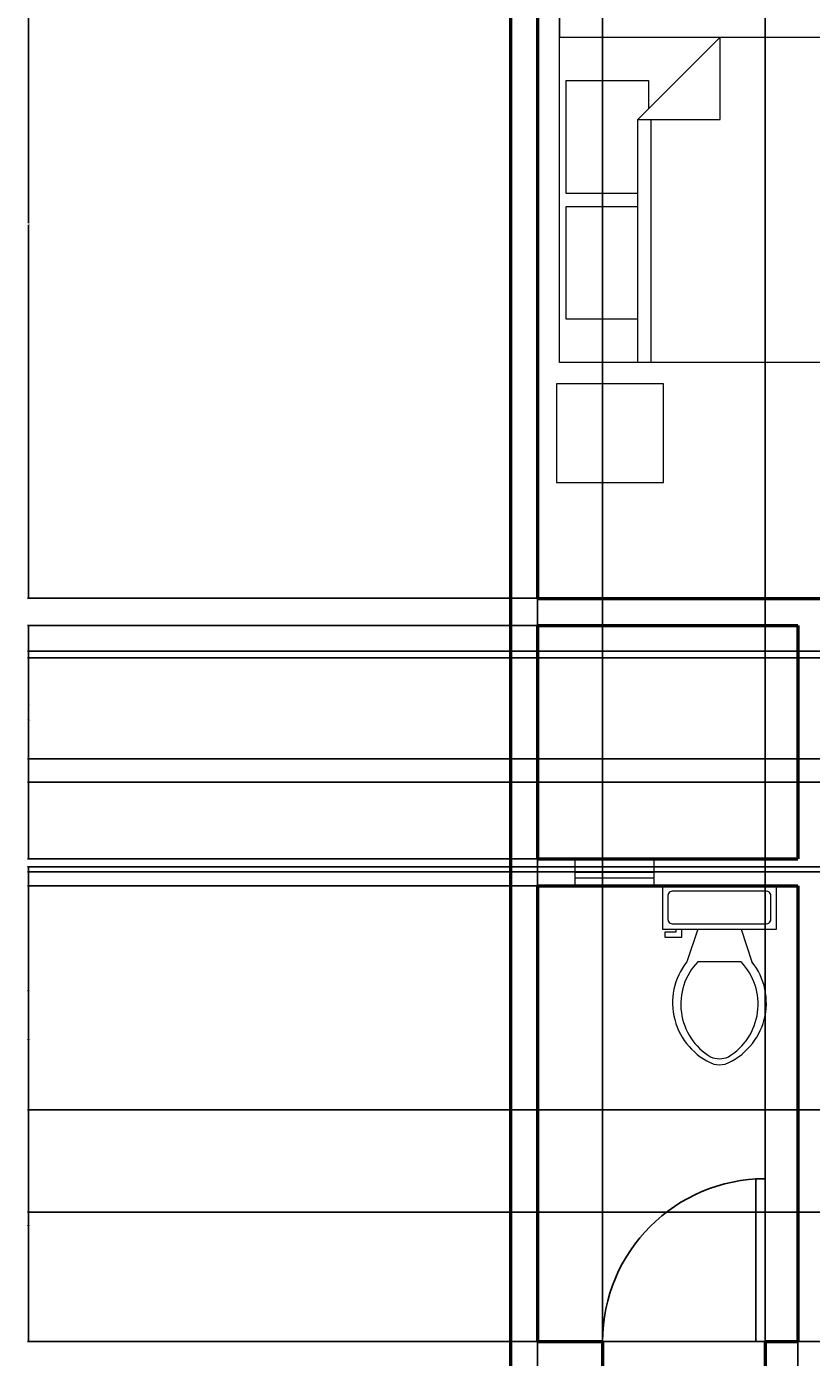
# Model space of a CAD drawing. Units: inches. Extents: x 115999 to 116502, y 188991 to 189729.
# Tile 2 of 5: x 115999 to 116144, y 189347 to 189592. Entities that reach past the tile are written whole.
import ezdxf

# ---------------------------------------------------------------- set-up
doc = ezdxf.new("R2010")
doc.units = ezdxf.units.IN
for name, color, linetype, lineweight in [('A-ANNO-DIMS', 2, 'Continuous', 18), ('A-DOOR', 4, 'Continuous', 25), ('A-FLOR-FIXT', 9, 'Continuous', 20), ('A-FURN', 8, 'Continuous', 18), ('A-GLAZ', 4, 'Continuous', 18), ('A-WALL', 7, 'Continuous', 50)]:
    doc.layers.add(name, color=color, linetype=linetype, lineweight=lineweight)
doc.styles.get("Standard").update_dxf_attribs({"font": 'arial.ttf'})
doc.dimstyles.get("Standard").update_dxf_attribs({"dimtxt": 0.18, "dimasz": 0.18, "dimexe": 0.18, "dimexo": 0.0625, "dimgap": 0.09, "dimtad": 0, "dimtih": 1, "dimtoh": 1, "dimdec": 4, "dimzin": 0, "dimdsep": 46, "dimtxsty": 'Standard', "dimcen": 0.09, "dimadec": 0, "dimazin": 0, "dimtfac": 1, "dimtdec": 4, "dimtofl": 0, "dimtmove": 0, "dimatfit": 3, "dimfxl": 1, "dimtolj": 1, "dimtzin": 0, "dimarcsym": 0})

# ---------------------------------------------------------------- blocks, each defined once
blk = doc.blocks.new('Toilet - top')
for p, q in [((9.5, -6), (9.5, -2)), ((-10, -8.5), (-8, -8.5)), ((-10, -9.5), (-10, -8.5)), ((-7, -9.5), (-10, -9.5)), ((-8, -8.5), (-8, -8)), ((-7, -8), (-7, -9.5)), ((-4, -8), (-6, -14)), ((4, -8), (6, -14)), ((4, -14), (-4, -14))]:
    blk.add_line(p, q)
blk.add_lwpolyline([(10.5, -8), (10.5, 0), (-10.5, 0), (-10.5, -8)], close=True)
for points in [[(-9.5, -2), (-9.5, -6)], [(8.5, -1), (-8.5, -1)], [(-8.5, -7), (8.5, -7)]]:
    blk.add_lwpolyline(points)
for centre, radius, start, end in [((-8.62, -1.88), 0.884, 81.8699, 188.1301), ((8.62, -1.88), 0.884, 351.8699, 98.1301), ((-8.62, -6.12), 0.884, 171.8699, 278.1301), ((8.62, -6.12), 0.884, 261.8699, 8.1301), ((3.52, -21.58), 12.17, 141.4691, 247.9714), ((4.2, -21.82), 11.33, 136.3677, 238.9468), ((-3.52, -21.58), 12.17, 292.0284, 38.5307), ((-4.2, -21.82), 11.33, 301.053, 43.6321), ((0, -27.88), 4, 245.7318, 294.2682), ((0, -29), 4, 254.8605, 285.1395)]:
    blk.add_arc(centre, radius, start, end)
blk = doc.blocks.new('Bed - Queen')
for p, q in [((0, -80.00003), (0, 0)), ((0, 0), (59.99999, 0)), ((59.99999, 0), (59.99999, -80.00003)), ((7.99999, -1.2), (28.79998, -1.2)), ((7.99999, -14.4), (7.99999, -1.2)), ((28.79998, -1.2), (28.79998, -14.4)), ((31.19999, -1.2), (51.99999, -1.2)), ((31.19999, -14.4), (31.19999, -1.2)), ((51.99999, -1.2), (51.99999, -16.4)), ((0, -14.4), (44.8, -14.4)), ((59.99999, -29.6), (44.8, -14.4)), ((44.8, -14.4), (44.8, -29.6)), ((44.8, -16.8), (0, -16.8)), ((51.99999, -16.4), (46.79936, -16.4)), ((44.8, -29.6), (59.99999, -29.6)), ((59.99999, -80.00003), (0, -80.00003))]:
    blk.add_line(p, q)
blk = doc.blocks.new('*U3')
for p, q in [((0, 0), (0, -5)), ((30, 0), (30, -5))]:
    blk.add_line(p, q)
blk.add_lwpolyline([(0, 0), (0, 30), (1.75, 30), (1.75, 0)], close=True)
blk.add_arc((0, 0), 30, 0, 90)
blk = doc.blocks.new('TABLE-NIGHTSTAND')
blk.add_lwpolyline([(0, 18.2), (19.71, 18.2), (19.71, 0), (0, 0)], close=True)
blk = doc.blocks.new('*D21')
at = {"layer": 'A-ANNO-DIMS', "color": 0, "lineweight": -2, "transparency": 16777216}
for p, q in [((116097.14, 189590.46), (116097.14, 189602.58)), ((116097.32, 189602.4), (116135.84, 189602.4)), ((116176.96, 189602.4), (116138.45, 189602.4)), ((116177.14, 189590.46), (116177.14, 189602.58))]:
    blk.add_line(p, q, dxfattribs=at)
at = {"layer": 'A-ANNO-DIMS', "color": 0, "transparency": 16777216}
for points in [[(116097.32, 189602.43), (116097.32, 189602.37), (116097.14, 189602.4)], [(116176.96, 189602.43), (116176.96, 189602.37), (116177.14, 189602.4)]]:
    blk.add_solid(points, dxfattribs=at)
at = {"layer": 'Defpoints', "color": 0, "transparency": 16777216}
for p in [(116097.14, 189602.4), (116097.14, 189590.4), (116177.14, 189590.4)]:
    blk.add_point(p, dxfattribs=at)
at = {"layer": 'A-ANNO-DIMS', "color": 0, "transparency": 16777216, "insert": (116137.14, 189602.4), "char_height": 0.18, "attachment_point": 5}
blk.add_mtext('\\A1;QUEEN BED 80 TYP.', dxfattribs=at)
blk = doc.blocks.new('*D33')
at = {"layer": 'A-ANNO-DIMS', "color": 0, "lineweight": -2, "transparency": 16777216}
for p, q in [((116088.06, 189088.01), (116088.06, 189728.73)), ((116088.24, 189728.55), (116277.77, 189728.55)), ((116467.88, 189728.55), (116278.35, 189728.55)), ((116468.06, 189088.01), (116468.06, 189728.73))]:
    blk.add_line(p, q, dxfattribs=at)
at = {"layer": 'A-ANNO-DIMS', "color": 0, "transparency": 16777216}
for points in [[(116088.24, 189728.58), (116088.24, 189728.52), (116088.06, 189728.55)], [(116467.88, 189728.58), (116467.88, 189728.52), (116468.06, 189728.55)]]:
    blk.add_solid(points, dxfattribs=at)
at = {"layer": 'Defpoints', "color": 0, "transparency": 16777216}
for p in [(116468.06, 189728.55), (116088.06, 189087.95), (116468.06, 189087.95)]:
    blk.add_point(p, dxfattribs=at)
at = {"layer": 'A-ANNO-DIMS', "color": 0, "transparency": 16777216, "insert": (116278.06, 189728.55), "char_height": 0.18, "attachment_point": 5}
blk.add_mtext('\\A1;380', dxfattribs=at)
blk = doc.blocks.new('*D39')
at = {"layer": 'A-ANNO-DIMS', "color": 0, "lineweight": -2, "transparency": 16777216}
for p, q in [((116093, 189624.95), (115999.04, 189624.95)), ((115999.22, 189624.77), (115999.22, 189556.13)), ((115999.22, 189487.13), (115999.22, 189555.76)), ((116093, 189486.95), (115999.04, 189486.95))]:
    blk.add_line(p, q, dxfattribs=at)
at = {"layer": 'A-ANNO-DIMS', "color": 0, "transparency": 16777216}
for points in [[(115999.19, 189624.77), (115999.25, 189624.77), (115999.22, 189624.95)], [(115999.19, 189487.13), (115999.25, 189487.13), (115999.22, 189486.95)]]:
    blk.add_solid(points, dxfattribs=at)
at = {"layer": 'Defpoints', "color": 0, "transparency": 16777216}
for p in [(115999.22, 189624.95), (116093.06, 189624.95), (116093.06, 189486.95)]:
    blk.add_point(p, dxfattribs=at)
at = {"layer": 'A-ANNO-DIMS', "color": 0, "transparency": 16777216, "insert": (115999.22, 189555.95), "char_height": 0.18, "attachment_point": 5}
blk.add_mtext('\\A1;138', dxfattribs=at)
blk = doc.blocks.new('*D41')
at = {"layer": 'A-ANNO-DIMS', "color": 0, "lineweight": -2, "transparency": 16777216}
for p, q in [((116093, 189433.95), (115999.04, 189433.95)), ((115999.22, 189433.77), (115999.22, 189392.13)), ((115999.22, 189350.13), (115999.22, 189391.77)), ((116093, 189349.95), (115999.04, 189349.95))]:
    blk.add_line(p, q, dxfattribs=at)
at = {"layer": 'A-ANNO-DIMS', "color": 0, "transparency": 16777216}
for points in [[(115999.19, 189433.77), (115999.25, 189433.77), (115999.22, 189433.95)], [(115999.19, 189350.13), (115999.25, 189350.13), (115999.22, 189349.95)]]:
    blk.add_solid(points, dxfattribs=at)
at = {"layer": 'Defpoints', "color": 0, "transparency": 16777216}
for p in [(115999.22, 189433.95), (116093.06, 189433.95), (116093.06, 189349.95)]:
    blk.add_point(p, dxfattribs=at)
at = {"layer": 'A-ANNO-DIMS', "color": 0, "transparency": 16777216, "insert": (115999.22, 189391.95), "char_height": 0.18, "attachment_point": 5}
blk.add_mtext('\\A1;84', dxfattribs=at)
blk = doc.blocks.new('*D42')
at = {"layer": 'A-ANNO-DIMS', "color": 0, "lineweight": -2, "transparency": 16777216}
for p, q in [((116093, 189481.95), (115999.04, 189481.95)), ((115999.22, 189481.77), (115999.22, 189460.63)), ((115999.22, 189439.13), (115999.22, 189460.26)), ((116093, 189438.95), (115999.04, 189438.95))]:
    blk.add_line(p, q, dxfattribs=at)
at = {"layer": 'A-ANNO-DIMS', "color": 0, "transparency": 16777216}
for points in [[(115999.19, 189481.77), (115999.25, 189481.77), (115999.22, 189481.95)], [(115999.19, 189439.13), (115999.25, 189439.13), (115999.22, 189438.95)]]:
    blk.add_solid(points, dxfattribs=at)
at = {"layer": 'Defpoints', "color": 0, "transparency": 16777216}
for p in [(115999.22, 189481.95), (116093.06, 189481.95), (116093.06, 189438.95)]:
    blk.add_point(p, dxfattribs=at)
at = {"layer": 'A-ANNO-DIMS', "color": 0, "transparency": 16777216, "insert": (115999.22, 189460.45), "char_height": 0.18, "attachment_point": 5}
blk.add_mtext('\\A1;43', dxfattribs=at)
blk = doc.blocks.new('*D43')
at = {"layer": 'A-ANNO-DIMS', "color": 0, "lineweight": -2, "transparency": 16777216}
for p, q in [((116093.06, 189624.88), (116093.06, 188991.26)), ((116272.06, 189624.88), (116272.06, 188991.26)), ((116093.24, 188991.44), (116182.28, 188991.44)), ((116271.88, 188991.44), (116182.84, 188991.44))]:
    blk.add_line(p, q, dxfattribs=at)
at = {"layer": 'A-ANNO-DIMS', "color": 0, "transparency": 16777216}
for points in [[(116093.24, 188991.47), (116093.24, 188991.41), (116093.06, 188991.44)], [(116271.88, 188991.47), (116271.88, 188991.41), (116272.06, 188991.44)]]:
    blk.add_solid(points, dxfattribs=at)
at = {"layer": 'Defpoints', "color": 0, "transparency": 16777216}
for p in [(116093.06, 189624.95), (116272.06, 189624.95), (116272.06, 188991.44)]:
    blk.add_point(p, dxfattribs=at)
at = {"layer": 'A-ANNO-DIMS', "color": 0, "transparency": 16777216, "insert": (116182.56, 188991.44), "char_height": 0.18, "attachment_point": 5}
blk.add_mtext('\\A1;179', dxfattribs=at)
blk = doc.blocks.new('*D51')
at = {"layer": 'A-ANNO-DIMS', "color": 0, "lineweight": -2, "transparency": 16777216}
for p, q in [((116093.06, 189349.88), (116093.06, 188991.26)), ((116141.06, 189349.88), (116141.06, 188991.26)), ((116093.24, 188991.44), (116116.84, 188991.44)), ((116140.88, 188991.44), (116117.29, 188991.44))]:
    blk.add_line(p, q, dxfattribs=at)
at = {"layer": 'A-ANNO-DIMS', "color": 0, "transparency": 16777216}
for points in [[(116093.24, 188991.47), (116093.24, 188991.41), (116093.06, 188991.44)], [(116140.88, 188991.47), (116140.88, 188991.41), (116141.06, 188991.44)]]:
    blk.add_solid(points, dxfattribs=at)
at = {"layer": 'Defpoints', "color": 0, "transparency": 16777216}
for p in [(116093.06, 189349.95), (116141.06, 189349.95), (116141.06, 188991.44)]:
    blk.add_point(p, dxfattribs=at)
at = {"layer": 'A-ANNO-DIMS', "color": 0, "transparency": 16777216, "insert": (116117.06, 188991.44), "char_height": 0.18, "attachment_point": 5}
blk.add_mtext('\\A1;48', dxfattribs=at)
blk = doc.blocks.new('*D53')
at = {"layer": 'A-ANNO-DIMS', "color": 0, "lineweight": -2, "transparency": 16777216}
for p, q in [((116331, 189436.5), (115999.04, 189436.5)), ((115999.22, 189436.32), (115999.22, 189414.77)), ((115999.22, 189392.85), (115999.22, 189414.41)), ((116331, 189392.67), (115999.04, 189392.67))]:
    blk.add_line(p, q, dxfattribs=at)
at = {"layer": 'A-ANNO-DIMS', "color": 0, "transparency": 16777216}
for points in [[(115999.19, 189436.32), (115999.25, 189436.32), (115999.22, 189436.5)], [(115999.19, 189392.85), (115999.25, 189392.85), (115999.22, 189392.67)]]:
    blk.add_solid(points, dxfattribs=at)
at = {"layer": 'Defpoints', "color": 0, "transparency": 16777216}
for p in [(115999.22, 189436.5), (116331.06, 189436.5), (116331.06, 189392.67)]:
    blk.add_point(p, dxfattribs=at)
at = {"layer": 'A-ANNO-DIMS', "color": 0, "transparency": 16777216, "insert": (115999.22, 189414.59), "char_height": 0.18, "attachment_point": 5}
blk.add_mtext('\\A1;43.83', dxfattribs=at)
blk = doc.blocks.new('*D55')
at = {"layer": 'A-ANNO-DIMS', "color": 0, "lineweight": -2, "transparency": 16777216}
for p, q in [((116266.44, 189437.45), (115999.04, 189437.45)), ((115999.22, 189437.27), (115999.22, 189405.79)), ((115999.22, 189373.95), (115999.22, 189405.43)), ((116266.44, 189373.77), (115999.04, 189373.77))]:
    blk.add_line(p, q, dxfattribs=at)
at = {"layer": 'A-ANNO-DIMS', "color": 0, "transparency": 16777216}
for points in [[(115999.19, 189437.27), (115999.25, 189437.27), (115999.22, 189437.45)], [(115999.19, 189373.95), (115999.25, 189373.95), (115999.22, 189373.77)]]:
    blk.add_solid(points, dxfattribs=at)
at = {"layer": 'Defpoints', "color": 0, "transparency": 16777216}
for p in [(115999.22, 189437.45), (116266.5, 189437.45), (116266.5, 189373.77)]:
    blk.add_point(p, dxfattribs=at)
at = {"layer": 'A-ANNO-DIMS', "color": 0, "transparency": 16777216, "insert": (115999.22, 189405.61), "char_height": 0.18, "attachment_point": 5}
blk.add_mtext('\\A1;63.68', dxfattribs=at)
blk = doc.blocks.new('*D67')
at = {"layer": 'A-ANNO-DIMS', "color": 0, "lineweight": -2, "transparency": 16777216}
for p, q in [((116331, 189392.67), (115999.04, 189392.67)), ((115999.22, 189392.49), (115999.22, 189371.49)), ((115999.22, 189350.13), (115999.22, 189371.13)), ((116331, 189349.95), (115999.04, 189349.95))]:
    blk.add_line(p, q, dxfattribs=at)
at = {"layer": 'A-ANNO-DIMS', "color": 0, "transparency": 16777216}
for points in [[(115999.19, 189392.49), (115999.25, 189392.49), (115999.22, 189392.67)], [(115999.19, 189350.13), (115999.25, 189350.13), (115999.22, 189349.95)]]:
    blk.add_solid(points, dxfattribs=at)
at = {"layer": 'Defpoints', "color": 0, "transparency": 16777216}
for p in [(115999.22, 189392.67), (116331.06, 189392.67), (116331.06, 189349.95)]:
    blk.add_point(p, dxfattribs=at)
at = {"layer": 'A-ANNO-DIMS', "color": 0, "transparency": 16777216, "insert": (115999.22, 189371.31), "char_height": 0.18, "attachment_point": 5}
blk.add_mtext('\\A1;42.73', dxfattribs=at)
blk = doc.blocks.new('*D70')
at = {"layer": 'A-ANNO-DIMS', "color": 0, "lineweight": -2, "transparency": 16777216}
for p, q in [((116105.06, 189350.01), (116105.06, 189728.73)), ((116105.24, 189728.55), (116119.84, 189728.55)), ((116134.88, 189728.55), (116120.28, 189728.55)), ((116135.06, 189350.01), (116135.06, 189728.73))]:
    blk.add_line(p, q, dxfattribs=at)
at = {"layer": 'A-ANNO-DIMS', "color": 0, "transparency": 16777216}
for points in [[(116105.24, 189728.58), (116105.24, 189728.52), (116105.06, 189728.55)], [(116134.88, 189728.58), (116134.88, 189728.52), (116135.06, 189728.55)]]:
    blk.add_solid(points, dxfattribs=at)
at = {"layer": 'Defpoints', "color": 0, "transparency": 16777216}
for p in [(116135.06, 189728.55), (116105.06, 189349.95), (116135.06, 189349.95)]:
    blk.add_point(p, dxfattribs=at)
at = {"layer": 'A-ANNO-DIMS', "color": 0, "transparency": 16777216, "insert": (116120.06, 189728.55), "char_height": 0.18, "attachment_point": 5}
blk.add_mtext('\\A1;30', dxfattribs=at)
blk = doc.blocks.new('*D73')
at = {"layer": 'A-ANNO-DIMS', "color": 0, "lineweight": -2, "transparency": 16777216}
for p, q in [((116093.06, 189350.01), (116093.06, 189728.73)), ((116093.24, 189728.55), (116098.85, 189728.55)), ((116104.88, 189728.55), (116099.27, 189728.55)), ((116105.06, 189350.01), (116105.06, 189728.73))]:
    blk.add_line(p, q, dxfattribs=at)
at = {"layer": 'A-ANNO-DIMS', "color": 0, "transparency": 16777216}
for points in [[(116093.24, 189728.58), (116093.24, 189728.52), (116093.06, 189728.55)], [(116104.88, 189728.58), (116104.88, 189728.52), (116105.06, 189728.55)]]:
    blk.add_solid(points, dxfattribs=at)
at = {"layer": 'Defpoints', "color": 0, "transparency": 16777216}
for p in [(116105.06, 189728.55), (116093.06, 189349.95), (116105.06, 189349.95)]:
    blk.add_point(p, dxfattribs=at)
at = {"layer": 'A-ANNO-DIMS', "color": 0, "transparency": 16777216, "insert": (116099.06, 189728.55), "char_height": 0.18, "attachment_point": 5}
blk.add_mtext('\\A1;12', dxfattribs=at)
blk = doc.blocks.new('*D81')
at = {"layer": 'A-ANNO-DIMS', "color": 0, "lineweight": -2, "transparency": 16777216}
for p, q in [((116185.46, 189475.99), (115999.04, 189475.99)), ((115999.22, 189475.81), (115999.22, 189464.71)), ((115999.22, 189453.24), (115999.22, 189464.34)), ((116188.46, 189453.06), (115999.04, 189453.06))]:
    blk.add_line(p, q, dxfattribs=at)
at = {"layer": 'A-ANNO-DIMS', "color": 0, "transparency": 16777216}
for points in [[(115999.19, 189475.81), (115999.25, 189475.81), (115999.22, 189475.99)], [(115999.19, 189453.24), (115999.25, 189453.24), (115999.22, 189453.06)]]:
    blk.add_solid(points, dxfattribs=at)
at = {"layer": 'Defpoints', "color": 0, "transparency": 16777216}
for p in [(116185.52, 189475.99), (115999.22, 189453.06), (116188.52, 189453.06)]:
    blk.add_point(p, dxfattribs=at)
at = {"layer": 'A-ANNO-DIMS', "color": 0, "transparency": 16777216, "insert": (115999.22, 189464.52), "char_height": 0.18, "attachment_point": 5}
blk.add_mtext('\\A1;22.926', dxfattribs=at)
blk = doc.blocks.new('*D83')
at = {"layer": 'A-ANNO-DIMS', "color": 0, "lineweight": -2, "transparency": 16777216}
for p, q in [((116152.34, 189477.21), (115999.04, 189477.21)), ((115999.22, 189477.03), (115999.22, 189467.47)), ((115999.22, 189457.56), (115999.22, 189467.11)), ((116152.34, 189457.38), (115999.04, 189457.38))]:
    blk.add_line(p, q, dxfattribs=at)
at = {"layer": 'A-ANNO-DIMS', "color": 0, "transparency": 16777216}
for points in [[(115999.19, 189477.03), (115999.25, 189477.03), (115999.22, 189477.21)], [(115999.19, 189457.56), (115999.25, 189457.56), (115999.22, 189457.38)]]:
    blk.add_solid(points, dxfattribs=at)
at = {"layer": 'Defpoints', "color": 0, "transparency": 16777216}
for p in [(115999.22, 189477.21), (116152.4, 189477.21), (116152.4, 189457.38)]:
    blk.add_point(p, dxfattribs=at)
at = {"layer": 'A-ANNO-DIMS', "color": 0, "transparency": 16777216, "insert": (115999.22, 189467.29), "char_height": 0.18, "attachment_point": 5}
blk.add_mtext('\\A1;19.83', dxfattribs=at)

msp = doc.modelspace()

# ---------------------------------------------------------------- linework, layer by layer
at = {"layer": 'A-GLAZ'}
for p, q in [((116099.919, 189438.9469), (116099.919, 189433.9469)), ((116114.5054, 189438.9469), (116114.5054, 189433.9469)), ((116099.919, 189437.4469), (116114.5054, 189437.4469)), ((116099.919, 189436.4469), (116114.5054, 189436.4469)), ((116099.919, 189435.4469), (116114.5054, 189435.4469))]:
    msp.add_line(p, q, dxfattribs=at)
at = {"layer": 'A-WALL'}
for p, q in [((116088.0631, 189694.9469), (116088.0631, 189087.9469)), ((116093.0631, 189624.9469), (116093.0631, 189486.9469)), ((116093.0631, 189486.9469), (116224.0631, 189486.9469)), ((116093.0631, 189481.9469), (116141.0631, 189481.9469)), ((116093.0631, 189481.9469), (116093.0631, 189438.9469)), ((116141.0631, 189481.9469), (116141.0631, 189438.9469)), ((116093.0631, 189438.9469), (116141.0631, 189438.9469)), ((116093.0631, 189433.9469), (116141.0631, 189433.9469)), ((116093.0631, 189433.9469), (116093.0631, 189349.9469)), ((116141.0631, 189433.9469), (116141.0631, 189349.9469)), ((116093.0631, 189349.9469), (116105.0631, 189349.9469)), ((116105.0631, 189349.9469), (116105.0631, 189344.9469)), ((116135.0631, 189349.9469), (116135.0631, 189344.9469)), ((116135.0631, 189349.9469), (116141.0631, 189349.9469))]:
    msp.add_line(p, q, dxfattribs=at)

# ---------------------------------------------------------------- block references
at = {"layer": 'A-DOOR', "xscale": -1}
msp.add_blockref('*U3', (116135.0631, 189349.9469), dxfattribs=at)
at = {"layer": 'A-FLOR-FIXT'}
msp.add_blockref('Toilet - top', (116126.6102, 189433.9469), dxfattribs=at)
at = {"layer": 'A-FURN', "rotation": 90}
msp.add_blockref('Bed - Queen', (116097.142, 189530.3971), dxfattribs=at)
at = {"layer": 'A-FURN', "extrusion": (0, 0, -1), "zscale": -1, "rotation": 180}
msp.add_blockref('TABLE-NIGHTSTAND', (-116096.5803, 189526.497), dxfattribs=at)

# ---------------------------------------------------------------- dimensions: what is measured, and where the dimension line sits
at = {"layer": 'A-ANNO-DIMS'}
for base, p1, p2, picture, middle in [((116468.0631, 189728.5469), (116088.0631, 189087.9469), (116468.0631, 189087.9469), '*D33', (116278.0631, 189728.5469)), ((116105.0631, 189728.5469), (116093.0631, 189349.9469), (116105.0631, 189349.9469), '*D73', (116099.0631, 189728.5469)), ((116135.0631, 189728.5469), (116105.0631, 189349.9469), (116135.0631, 189349.9469), '*D70', (116120.0631, 189728.5469)), ((116272.0631, 188991.4393), (116093.0631, 189624.9469), (116272.0631, 189624.9469), '*D43', (116182.5631, 188991.4393)), ((116141.0631, 188991.4393), (116093.0631, 189349.9469), (116141.0631, 189349.9469), '*D51', (116117.0631, 188991.4393))]:
    dim = msp.add_linear_dim(base=base, p1=p1, p2=p2, dimstyle='Standard', override={"dimdec": 0, "dimlfac": 1, "dimrnd": 0, "dimzin": 0, "dimdsep": 46, "dimlunit": 2}, dxfattribs=at)
    dim.commit()
    dim.dimension.update_dxf_attribs({"geometry": picture, "text_midpoint": middle})
for base, p1, p2, override, picture, middle in [((115999.2211, 189624.9469), (116093.0631, 189486.9469), (116093.0631, 189624.9469), {"dimdec": 0, "dimlfac": 1, "dimrnd": 0, "dimzin": 0, "dimdsep": 46, "dimlunit": 2}, '*D39', (115999.2211, 189555.9469)), ((115999.2211, 189481.9469), (116093.0631, 189438.9469), (116093.0631, 189481.9469), {"dimdec": 0, "dimlfac": 1, "dimrnd": 0, "dimzin": 0, "dimdsep": 46, "dimlunit": 2}, '*D42', (115999.2211, 189460.4469)), ((115999.2211, 189453.0603), (116185.5193, 189475.9866), (116188.5186, 189453.0603), {"dimdec": 3, "dimlfac": 1, "dimrnd": 0, "dimzin": 0, "dimdsep": 46, "dimlunit": 2}, '*D81', (115999.2211, 189464.5234)), ((115999.2211, 189477.2058), (116152.4048, 189457.376), (116152.4048, 189477.2058), {"dimdec": 2, "dimlfac": 1, "dimrnd": 0, "dimzin": 0, "dimdsep": 46, "dimlunit": 2}, '*D83', (115999.2211, 189467.2909)), ((115999.2211, 189437.4482), (116266.5001, 189373.7675), (116266.5001, 189437.4482), {"dimdec": 2, "dimlfac": 1, "dimrnd": 0, "dimzin": 0, "dimdsep": 46, "dimlunit": 2}, '*D55', (115999.2211, 189405.6079)), ((115999.2211, 189436.5016), (116331.0631, 189392.6745), (116331.0631, 189436.5016), {"dimdec": 2, "dimlfac": 1, "dimrnd": 0, "dimzin": 0, "dimdsep": 46, "dimlunit": 2}, '*D53', (115999.2211, 189414.588)), ((115999.2211, 189433.9469), (116093.0631, 189349.9469), (116093.0631, 189433.9469), {"dimdec": 0, "dimlfac": 1, "dimrnd": 0, "dimzin": 0, "dimdsep": 46, "dimlunit": 2}, '*D41', (115999.2211, 189391.9469)), ((115999.2211, 189392.6745), (116331.0631, 189349.9469), (116331.0631, 189392.6745), {"dimdec": 2, "dimlfac": 1, "dimrnd": 0, "dimzin": 0, "dimdsep": 46, "dimlunit": 2}, '*D67', (115999.2211, 189371.3107))]:
    dim = msp.add_linear_dim(base=base, p1=p1, p2=p2, angle=90, dimstyle='Standard', override=override, dxfattribs=at)
    dim.commit()
    dim.dimension.update_dxf_attribs({"geometry": picture, "text_midpoint": middle})
dim = msp.add_linear_dim(base=(116097.142, 189602.3971), p1=(116177.1421, 189590.397), p2=(116097.142, 189590.397), angle=180, text='QUEEN BED <> TYP.', dimstyle='Standard', override={"dimdec": 0, "dimlfac": 1, "dimrnd": 0, "dimzin": 0, "dimdsep": 46, "dimlunit": 2}, dxfattribs=at)
dim.commit()
dim.dimension.update_dxf_attribs({"geometry": '*D21', "text_midpoint": (116137.142, 189602.3971)})

doc.saveas('drawing.dxf')
